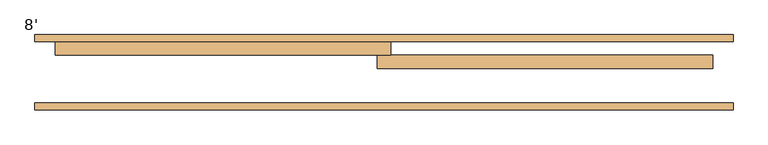
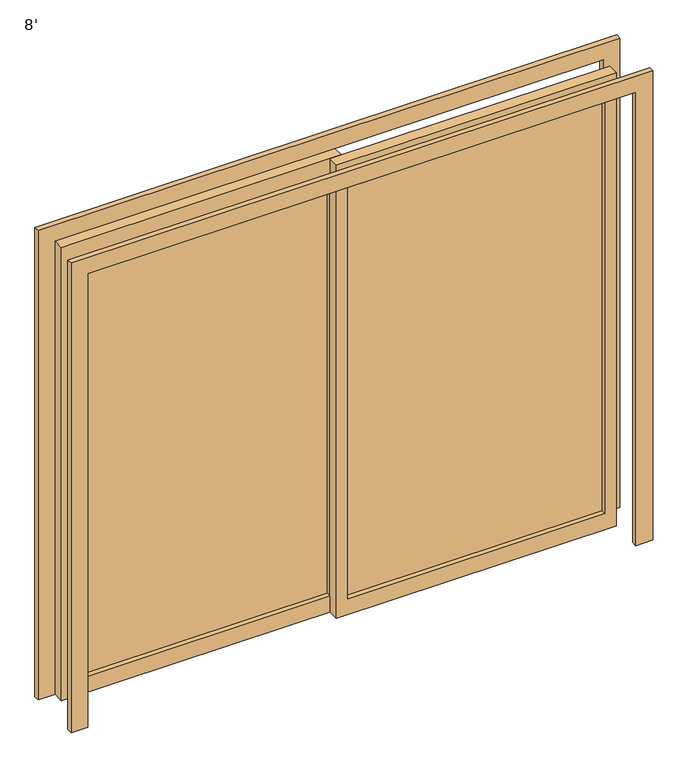
"""IFC4 building model written with IfcOpenShell, lengths in millimetres: door geometry, 8'."""

from ifc_helpers import new_model, si_unit, frame, origin, place, context, project, spatial, polyline, outline, extrude, source, transform, mapped, element, save


def door_8_4088deed(model_context):
    return source(origin(), model_context, "Body", "SweptSolid", [
        extrude(outline(polyline([(0.0, 1294.2), (2209.0, 1294.2), (2209.0, -1294.2), (0.0, -1294.2), (0.0, -1219.2), (2134.0, -1219.2), (2134.0, 1219.2), (0.0, 1219.2), (0.0, 1294.2)])), frame((0.0, 241.3, 0.0), z_axis=(0.0, 1.0, 0.0), x_axis=(0.0, 0.0, 1.0)), (0.0, 0.0, 1.0), 25.0),
        extrude(outline(polyline([(0.0, -1294.2), (0.0, -1219.2), (2134.0, -1219.2), (2134.0, 1219.2), (0.0, 1219.2), (0.0, 1294.2), (2209.0, 1294.2), (2209.0, -1294.2), (0.0, -1294.2)])), frame((0.0, -12.3, 0.0), z_axis=(0.0, 1.0, 0.0), x_axis=(0.0, 0.0, 1.0)), (0.0, 0.0, 1.0), 25.0),
        extrude(outline(polyline([(2134.0, 25.4), (2134.0, -1219.2), (0.0, -1219.2), (0.0, 25.4), (2134.0, 25.4)]), holes=[polyline([(2059.0, -24.6), (75.0, -24.6), (75.0, -1169.2), (2059.0, -1169.2), (2059.0, -24.6)])]), frame((0.0, 191.3, 0.0), z_axis=(0.0, 1.0, 0.0), x_axis=(0.0, 0.0, 1.0)), (0.0, 0.0, 1.0), 50.0),
        extrude(outline(polyline([(-1169.2, 219.475), (-24.6, 219.475), (-24.6, 213.125), (-1169.2, 213.125), (-1169.2, 219.475)])), frame((0.0, 0.0, 75.0), z_axis=(0.0, 0.0, 1.0), x_axis=(1.0, 0.0, 0.0)), (0.0, 0.0, 1.0), 1984.0),
        extrude(outline(polyline([(2134.0, -25.4), (0.0, -25.4), (0.0, 1219.2), (2134.0, 1219.2), (2134.0, -25.4)]), holes=[polyline([(2059.0, 24.6), (2059.0, 1169.2), (75.0, 1169.2), (75.0, 24.6), (2059.0, 24.6)])]), frame((0.0, 141.3, 0.0), z_axis=(0.0, 1.0, 0.0), x_axis=(0.0, 0.0, 1.0)), (0.0, 0.0, 1.0), 50.0),
        extrude(outline(polyline([(25.4, 169.475), (1169.2, 169.475), (1169.2, 163.125), (25.4, 163.125), (25.4, 169.475)])), frame((0.0, 0.0, 75.0), z_axis=(0.0, 0.0, 1.0), x_axis=(1.0, 0.0, 0.0)), (0.0, 0.0, 1.0), 1984.0),
    ])


if __name__ == "__main__":
    model = new_model("IFC4")
    model_context = context("Model", 3, world=origin())
    ifc_project = project(units=[si_unit("LENGTHUNIT", "METRE", prefix="MILLI")], contexts=[model_context])
    site = spatial("IfcSite", under=ifc_project)
    building = spatial("IfcBuilding", under=site)
    placement = place(None, origin())
    door_8_shape = door_8_4088deed(model_context)
    element("IfcDoor", 1, ObjectType="8'", at=placement, inside=building, context=model_context, shape_type="MappedRepresentation", body=[
        mapped(door_8_shape, transform((0.0, 0.0, 0.0), x_axis=(1.0, 0.0, 0.0), y_axis=(0.0, 1.0, 0.0), z_axis=(0.0, 0.0, 1.0))),
    ])
    save(model, "model.ifc")

# Revit data of these elements
# Type "8'"
#   Type Mark = "56"
#   Thickness = 0' - 1.9685"
#   Height = 7' - 0.01575"
#   Anchura de barandal = 0' - 2.95276"
#   Anchura de montante = 0' - 1.9685"
#   Proyección cubrejuntas ext. = 0' - 0.98425"
#   Proyección cubrejuntas int. = 0' - 0.98425"
#   Anchura de cubrejuntas = 0' - 2.95276"
#   Width = 8' - 0"
#   Material de puerta = Puerta - Panel
#   Function = (empty or 0)
#   Assembly Code = ""
#   Wall Closure = (empty or 0)
# Element 1 (IfcDoor, "8'")
#   Materials on its faces: "Puerta - Panel", "Cristal"
# Materials
#   "Puerta - Panel": class "Madera", colour RGB 210 159 95, transparency 0
#   "Cristal": class "Vidrio", colour RGB 0 0 255, transparency 0.75
